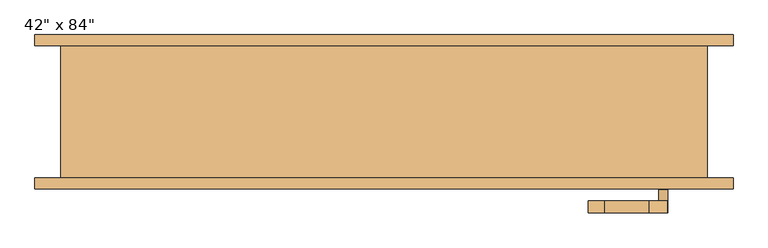
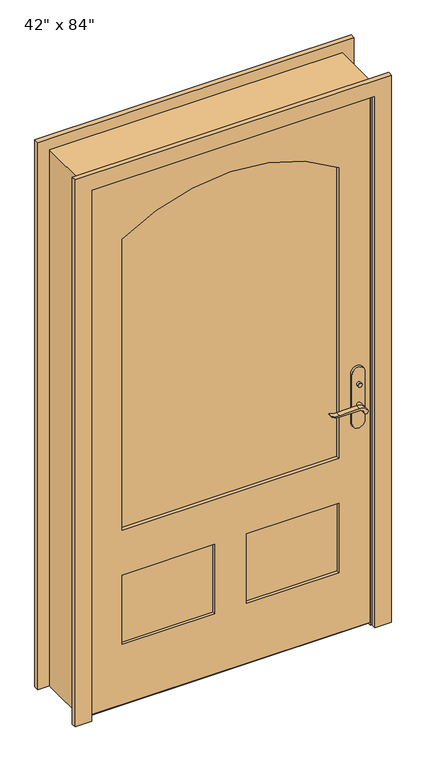
"""IFC4 building model written with IfcOpenShell, lengths in millimetres: door geometry."""

from ifc_helpers import new_model, si_unit, point, frame, frame_2d, origin, place, context, project, spatial, polyline, circle_curve, trimmed, segment, composite_curve, outline, extrude, faceted_brep, source, transform, mapped, element, save


def door_f44993c8(model_context):
    return source(origin(), model_context, "Body", "SolidModel", [
        extrude(outline(polyline([(-38.1, 12.7), (-12.7, 0.0), (-98.425, 0.0), (-73.025, 12.7), (-38.1, 12.7)])), frame((-533.4, 0.0, 0.0), z_axis=(1.0, 0.0, 0.0), x_axis=(0.0, 1.0, 0.0)), (0.0, 0.0, 1.0), 1066.8),
        extrude(outline(polyline([(487.6, -56.2), (487.6, -66.2), (477.6, -66.2), (477.6, -56.2), (487.6, -56.2)])), frame((0.0, 0.0, 981.9), z_axis=(0.0, 0.0, 1.0), x_axis=(1.0, 0.0, 0.0)), (0.0, 0.0, 1.0), 30.0),
        extrude(outline(composite_curve([segment(trimmed(circle_curve(frame_2d((996.9, 482.6)), 8.0), [point((996.9, 474.6))], [point((996.9, 490.6))], False, "CARTESIAN"), True, "CONTINUOUS"), segment(trimmed(circle_curve(frame_2d((996.9, 482.6)), 8.0), [point((996.9, 490.6))], [point((996.9, 474.6))], False, "CARTESIAN"), True, "CONTINUOUS")], self_intersect=False)), frame((0.0, -131.125, 0.0), z_axis=(0.0, 1.0, 0.0), x_axis=(0.0, 0.0, 1.0)), (0.0, 0.0, 1.0), 10.0),
        extrude(outline(composite_curve([segment(trimmed(circle_curve(frame_2d((897.1555521, 458.9324871)), 37.2832219), [point((919.0523287, 489.1081363))], [point((934.4, 457.2325667))], False, "CARTESIAN"), True, "CONTINUOUS"), segment(polyline([(934.4, 457.2325667), (934.4, 380.9564091)]), True, "CONTINUOUS"), segment(trimmed(circle_curve(frame_2d((1017.6850638, 381.0227909)), 83.2850902), [point((934.4, 380.9564091))], [point((939.4, 352.6))], True, "CARTESIAN"), True, "CONTINUOUS"), segment(polyline([(939.4, 352.6), (936.6135558, 352.6)]), True, "CONTINUOUS"), segment(trimmed(circle_curve(frame_2d((986.6709207, 384.5396612)), 59.3791355), [point((936.6135558, 352.6))], [point((927.4, 380.9564091))], False, "CARTESIAN"), True, "CONTINUOUS"), segment(polyline([(927.4, 380.9564091), (927.4, 457.2138099)]), True, "CONTINUOUS"), segment(trimmed(circle_curve(frame_2d((909.2738613, 457.2138099)), 18.1261387), [point((927.4, 457.2138099))], [point((914.4, 474.6))], True, "CARTESIAN"), True, "CONTINUOUS"), segment(trimmed(circle_curve(frame_2d((914.4, 482.6)), 8.0), [point((914.4, 474.6))], [point((919.0523287, 489.1081363))], False, "CARTESIAN"), True, "CONTINUOUS")], self_intersect=False)), frame((0.0, -36.2, 0.0), z_axis=(0.0, 1.0, 0.0), x_axis=(0.0, 0.0, 1.0)), (0.0, 0.0, 1.0), 20.0),
        extrude(outline(composite_curve([segment(trimmed(circle_curve(frame_2d((914.4, 482.6)), 8.0), [point((914.3999903, 474.6))], [point((919.0523287, 489.1081363))], False, "CARTESIAN"), True, "CONTINUOUS"), segment(trimmed(circle_curve(frame_2d((897.1555521, 458.9324871)), 37.2832219), [point((919.0523287, 489.1081363))], [point((934.4, 457.2325667))], False, "CARTESIAN"), True, "CONTINUOUS"), segment(polyline([(934.4, 457.2325667), (934.4, 380.9564091)]), True, "CONTINUOUS"), segment(trimmed(circle_curve(frame_2d((1017.6850638, 381.0227909)), 83.2850902), [point((934.4, 380.9564091))], [point((939.4, 352.6))], True, "CARTESIAN"), True, "CONTINUOUS"), segment(polyline([(939.4, 352.6), (936.6135558, 352.6)]), True, "CONTINUOUS"), segment(trimmed(circle_curve(frame_2d((986.6709207, 384.5396612)), 59.3791355), [point((936.6135558, 352.6))], [point((927.4, 380.9564091))], False, "CARTESIAN"), True, "CONTINUOUS"), segment(polyline([(927.4, 380.9564091), (927.4, 457.2138122)]), True, "CONTINUOUS"), segment(trimmed(circle_curve(frame_2d((909.2738682, 457.2138122)), 18.1261318), [point((927.4, 457.2138122))], [point((914.3999903, 474.6))], True, "CARTESIAN"), True, "CONTINUOUS")], self_intersect=False)), frame((0.0, -171.125, 0.0), z_axis=(0.0, 1.0, 0.0), x_axis=(0.0, 0.0, 1.0)), (0.0, 0.0, 1.0), 20.0),
        extrude(outline(composite_curve([segment(trimmed(circle_curve(frame_2d((914.4, 482.6)), 8.0), [point((914.4, 474.6))], [point((914.4, 490.6))], False, "CARTESIAN"), True, "CONTINUOUS"), segment(trimmed(circle_curve(frame_2d((914.4, 482.6)), 8.0), [point((914.4, 490.6))], [point((914.4, 474.6))], False, "CARTESIAN"), True, "CONTINUOUS")], self_intersect=False)), frame((0.0, -66.2, 0.0), z_axis=(0.0, 1.0, 0.0), x_axis=(0.0, 0.0, 1.0)), (0.0, 0.0, 1.0), 30.0),
        extrude(outline(composite_curve([segment(trimmed(circle_curve(frame_2d((914.4, 482.6)), 8.0), [point((914.4, 474.6))], [point((914.4, 490.6))], False, "CARTESIAN"), True, "CONTINUOUS"), segment(trimmed(circle_curve(frame_2d((914.4, 482.6)), 8.0), [point((914.4, 490.6))], [point((914.4, 474.6))], False, "CARTESIAN"), True, "CONTINUOUS")], self_intersect=False)), frame((0.0, -151.125, 0.0), z_axis=(0.0, 1.0, 0.0), x_axis=(0.0, 0.0, 1.0)), (0.0, 0.0, 1.0), 30.0),
        extrude(outline(composite_curve([segment(polyline([(844.4, 507.6), (1039.4, 507.6)]), True, "CONTINUOUS"), segment(trimmed(circle_curve(frame_2d((1039.4, 482.6)), 25.0), [point((1039.4, 507.6))], [point((1039.4, 457.6))], False, "CARTESIAN"), True, "CONTINUOUS"), segment(polyline([(1039.4, 457.6), (844.4, 457.6)]), True, "CONTINUOUS"), segment(trimmed(circle_curve(frame_2d((844.4, 482.6)), 25.0), [point((844.4, 457.6))], [point((844.4, 507.6))], False, "CARTESIAN"), True, "CONTINUOUS")], self_intersect=False)), frame((0.0, -76.2, 0.0), z_axis=(0.0, 1.0, 0.0), x_axis=(0.0, 0.0, 1.0)), (0.0, 0.0, 1.0), 10.0),
        extrude(outline(composite_curve([segment(polyline([(844.4, 507.6), (1039.4, 507.6)]), True, "CONTINUOUS"), segment(trimmed(circle_curve(frame_2d((1039.4, 482.6)), 25.0), [point((1039.4, 507.6))], [point((1039.4, 457.6))], False, "CARTESIAN"), True, "CONTINUOUS"), segment(polyline([(1039.4, 457.6), (844.4, 457.6)]), True, "CONTINUOUS"), segment(trimmed(circle_curve(frame_2d((844.4, 482.6)), 25.0), [point((844.4, 457.6))], [point((844.4, 507.6))], False, "CARTESIAN"), True, "CONTINUOUS")], self_intersect=False)), frame((0.0, -121.125, 0.0), z_axis=(0.0, 1.0, 0.0), x_axis=(0.0, 0.0, 1.0)), (0.0, 0.0, 1.0), 10.0),
        faceted_brep([(558.8, -111.125, 0.0), (533.4, -111.125, 0.0), (533.4, -76.2, 0.0), (520.7, -76.2, 0.0), (520.7, -41.275, 0.0), (533.4, -41.275, 0.0), (533.4, 117.475, 0.0), (558.8, 117.475, 0.0), (558.8, 117.475, 2159.0), (558.8, -111.125, 2159.0), (533.4, 117.475, 2133.6), (-533.4, 117.475, 2133.6), (-533.4, 117.475, 0.0), (-558.8, 117.475, 0.0), (-558.8, 117.475, 2159.0), (533.4, -41.275, 2133.6), (520.7, -41.275, 2120.9), (-520.7, -41.275, 2120.9), (-520.7, -41.275, 0.0), (-533.4, -41.275, 0.0), (-533.4, -41.275, 2133.6), (520.7, -76.2, 2120.9), (533.4, -76.2, 2133.6), (-533.4, -76.2, 2133.6), (-533.4, -76.2, 0.0), (-520.7, -76.2, 0.0), (-520.7, -76.2, 2120.9), (533.4, -111.125, 2133.6), (-558.8, -111.125, 2159.0), (-558.8, -111.125, 0.0), (-533.4, -111.125, 0.0), (-533.4, -111.125, 2133.6)], [[[0, 1, 2, 3, 4, 5, 6, 7]], [[7, 8, 9, 0]], [[6, 10, 11, 12, 13, 14, 8, 7]], [[5, 15, 10, 6]], [[4, 16, 17, 18, 19, 20, 15, 5]], [[3, 21, 16, 4]], [[2, 22, 23, 24, 25, 26, 21, 3]], [[1, 27, 22, 2]], [[0, 9, 28, 29, 30, 31, 27, 1]], [[8, 14, 28, 9]], [[15, 20, 11, 10]], [[21, 26, 17, 16]], [[27, 31, 23, 22]], [[29, 13, 12, 19, 18, 25, 24, 30]], [[14, 13, 29, 28]], [[20, 19, 12, 11]], [[26, 25, 18, 17]], [[31, 30, 24, 23]]]),
        extrude(outline(polyline([(2133.6, -533.4), (12.7, -533.4), (12.7, 533.4), (2133.6, 533.4), (2133.6, -533.4)]), holes=[composite_curve([segment(polyline([(714.375, -412.75), (1885.95, -412.75)]), True, "CONTINUOUS"), segment(trimmed(circle_curve(frame_2d((1278.73125, 0.0)), 734.21875), [point((1885.95, -412.75))], [point((1885.95, 412.75))], True, "CARTESIAN"), True, "CONTINUOUS"), segment(polyline([(1885.95, 412.75), (714.375, 412.75), (714.375, -412.75)]), True, "CONTINUOUS")], self_intersect=False), polyline([(533.4, -60.325), (254.0, -60.325), (254.0, -412.75), (533.4, -412.75), (533.4, -60.325)]), polyline([(533.4, 412.75), (254.0, 412.75), (254.0, 60.325), (533.4, 60.325), (533.4, 412.75)])]), frame((0.0, -111.125, 0.0), z_axis=(0.0, 1.0, 0.0), x_axis=(0.0, 0.0, 1.0)), (0.0, 0.0, 1.0), 34.925),
        extrude(outline(composite_curve([segment(polyline([(714.375, -412.75), (714.375, 412.75), (1885.95, 412.75)]), True, "CONTINUOUS"), segment(trimmed(circle_curve(frame_2d((1278.73125, 0.0)), 734.21875), [point((1885.95, 412.75))], [point((1885.95, -412.75))], False, "CARTESIAN"), True, "CONTINUOUS"), segment(polyline([(1885.95, -412.75), (714.375, -412.75)]), True, "CONTINUOUS")], self_intersect=False)), frame((0.0, -97.155, 0.0), z_axis=(0.0, 1.0, 0.0), x_axis=(0.0, 0.0, 1.0)), (0.0, 0.0, 1.0), 6.985),
        extrude(outline(polyline([(-60.325, -87.8416667), (-60.325, -99.4833333), (-412.75, -99.4833333), (-412.75, -87.8416667), (-60.325, -87.8416667)])), frame((0.0, 0.0, 254.0), z_axis=(0.0, 0.0, 1.0), x_axis=(1.0, 0.0, 0.0)), (0.0, 0.0, 1.0), 279.4),
        extrude(outline(polyline([(412.75, -87.8416667), (412.75, -99.4833333), (60.325, -99.4833333), (60.325, -87.8416667), (412.75, -87.8416667)])), frame((0.0, 0.0, 254.0), z_axis=(0.0, 0.0, 1.0), x_axis=(1.0, 0.0, 0.0)), (0.0, 0.0, 1.0), 279.4),
        extrude(outline(polyline([(0.0, -539.75), (2139.95, -539.75), (2139.95, 539.75), (0.0, 539.75), (0.0, 603.25), (2203.45, 603.25), (2203.45, -603.25), (0.0, -603.25), (0.0, -539.75)])), frame((0.0, -130.175, 0.0), z_axis=(0.0, 1.0, 0.0), x_axis=(0.0, 0.0, 1.0)), (0.0, 0.0, 1.0), 19.05),
        extrude(outline(polyline([(0.0, -539.75), (2139.95, -539.75), (2139.95, 539.75), (0.0, 539.75), (0.0, 603.25), (2203.45, 603.25), (2203.45, -603.25), (0.0, -603.25), (0.0, -539.75)])), frame((0.0, 117.475, 0.0), z_axis=(0.0, 1.0, 0.0), x_axis=(0.0, 0.0, 1.0)), (0.0, 0.0, 1.0), 19.05),
    ])


if __name__ == "__main__":
    model = new_model("IFC4")
    model_context = context("Model", 3, world=origin())
    ifc_project = project(units=[si_unit("LENGTHUNIT", "METRE", prefix="MILLI")], contexts=[model_context])
    site = spatial("IfcSite", under=ifc_project)
    building = spatial("IfcBuilding", under=site)
    placement = place(None, origin())
    door_shape = door_f44993c8(model_context)
    element("IfcDoor", 1, ObjectType="42\" x 84\"", at=placement, inside=building, context=model_context, shape_type="MappedRepresentation", body=[
        mapped(door_shape, transform((0.0, 0.0, 0.0), x_axis=(1.0, 0.0, 0.0), y_axis=(0.0, 1.0, 0.0), z_axis=(0.0, 0.0, 1.0))),
    ])
    save(model, "model.ifc")

# Revit data of these elements
# Type "42\" x 84\""
#   Type Mark = "11"
#   Assembly Code = "B2030100"
#   Analytic Construction = "French door, wood frame with single glass"
#   Threshold Offset [instance default] = 0' - 0 1/2"
#   Thickness = 0' - 1 3/8"
#   Thermal Resistance (R) = 1.0696 (h·ft²·°F)/BTU
#   Swing Angle [instance default] = 90.00°
#   Stiles = 0' - 4 3/4"
#   Rough Width = 3' - 8"
#   Rough Height = 7' - 1"
#   Radius = 2' - 4 29/32"
#   Lock Rail = 0' - 7 1/8"
#   Height = 7' - 0"
#   Width = 3' - 6"
#   Heat Transfer Coefficient (U) = 0.9350 BTU/(h·ft²·°F)
#   Door Offset [instance default] = 0' - 0"
#   Bottom Rail = 0' - 9 1/2"
#   Threshold [instance default] = yes
#   Function = 1
#   Exterior Trim [instance default] = yes
#   Trim Material = Cherry
#   Threshold Material = Cherry
#   Panel Material = Cherry
#   Glazing = Glass
#   Frame Material = Cherry
#   Door Handle Material = Aluminum
#   Visual Light Transmittance = 0
#   Solar Heat Gain Coefficient = 0
#   Wall Closure = (empty or 0)
#   Construction Type = (empty or 0)
# Element 1 (IfcDoor, "42\" x 84\"")
#   Materials on its faces: "Cherry", "Aluminum", "Glass"
# Materials
#   "Cherry": class "Wood", colour RGB 226 177 128, transparency 0, Description = "Prunus Serotina", Cost = 0
#   "Glass": class "Glass", colour RGB 0 128 192, transparency 0.75, Description = "Soda Lime Glass", Cost = 0
#   "Aluminum": class "Metal", colour RGB 247 247 247, transparency 0, Description = "Aluminum 6061", Cost = 0
